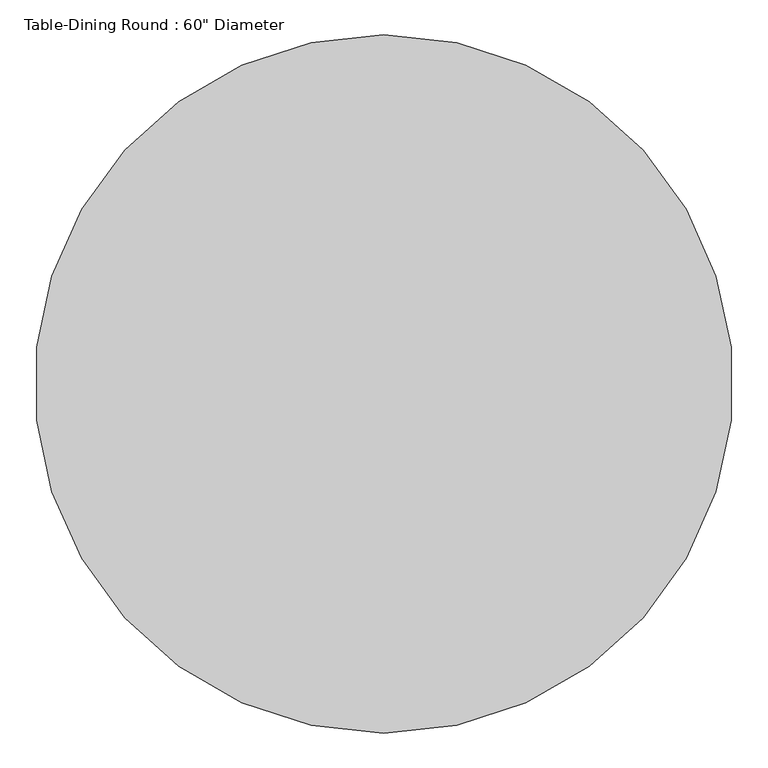
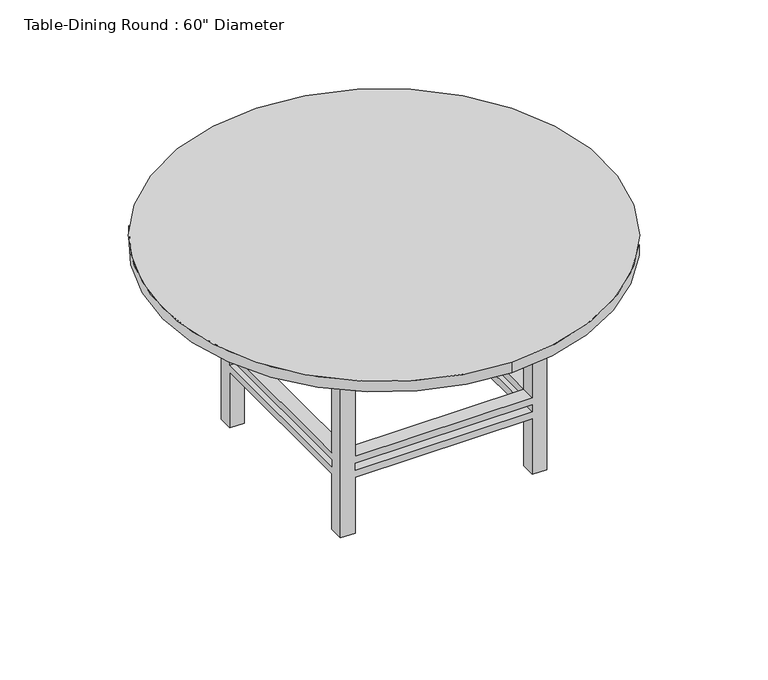
"""IFC4 building model written with IfcOpenShell, lengths in millimetres: furniture geometry."""

from ifc_helpers import new_model, si_unit, point, frame, frame_2d, origin, place, context, project, spatial, polyline, circle_curve, trimmed, segment, composite_curve, outline, extrude, faceted_brep, source, transform, mapped, element, save


def furniture_720490b2(model_context):
    return source(origin(), model_context, "Body", "SolidModel", [
        faceted_brep([(-201.1180328, 170.7213115, 723.9), (-251.9180328, 170.7213115, 723.9), (-251.9180328, 119.9213115, 723.9), (-201.1180328, 119.9213115, 723.9), (408.4819672, 170.7213115, 723.9), (408.4819672, 119.9213115, 723.9), (459.2819672, 119.9213115, 723.9), (459.2819672, 170.7213115, 723.9), (408.4819672, -540.4786885, 723.9), (459.2819672, -540.4786885, 723.9), (459.2819672, -489.6786885, 723.9), (408.4819672, -489.6786885, 723.9), (-201.1180328, -540.4786885, 723.9), (-201.1180328, -489.6786885, 723.9), (-251.9180328, -489.6786885, 723.9), (-251.9180328, -540.4786885, 723.9), (-201.1180328, 170.7213115, 0.0), (-201.1180328, 119.9213115, 0.0), (-251.9180328, 119.9213115, 0.0), (-251.9180328, 170.7213115, 0.0), (408.4819672, 170.7213115, 0.0), (459.2819672, 170.7213115, 0.0), (459.2819672, 119.9213115, 0.0), (408.4819672, 119.9213115, 0.0), (408.4819672, -540.4786885, 0.0), (408.4819672, -489.6786885, 0.0), (459.2819672, -489.6786885, 0.0), (459.2819672, -540.4786885, 0.0), (-201.1180328, -540.4786885, 0.0), (-251.9180328, -540.4786885, 0.0), (-251.9180328, -489.6786885, 0.0), (-201.1180328, -489.6786885, 0.0), (-201.1180328, 170.7213115, 279.4), (408.4819672, 170.7213115, 279.4), (408.4819672, 170.7213115, 203.2), (-201.1180328, 170.7213115, 203.2), (408.4819672, 170.7213115, 228.6), (408.4819672, 170.7213115, 254.0), (-201.1180328, 170.7213115, 254.0), (-201.1180328, 170.7213115, 228.6), (-251.9180328, 119.9213115, 203.2), (-251.9180328, -489.6786885, 203.2), (-251.9180328, -489.6786885, 279.4), (-251.9180328, 119.9213115, 279.4), (-251.9180328, 119.9213115, 228.6), (-251.9180328, 119.9213115, 254.0), (-251.9180328, -489.6786885, 254.0), (-251.9180328, -489.6786885, 228.6), (-201.1180328, 119.9213115, 279.4), (-201.1180328, 119.9213115, 203.2), (-201.1180328, 119.9213115, 228.6), (-201.1180328, 119.9213115, 254.0), (408.4819672, 119.9213115, 279.4), (408.4819672, 119.9213115, 203.2), (408.4819672, 119.9213115, 228.6), (408.4819672, 119.9213115, 254.0), (459.2819672, 119.9213115, 279.4), (459.2819672, 119.9213115, 203.2), (459.2819672, 119.9213115, 228.6), (459.2819672, 119.9213115, 254.0), (459.2819672, -489.6786885, 279.4), (459.2819672, -489.6786885, 203.2), (459.2819672, -489.6786885, 228.6), (459.2819672, -489.6786885, 254.0), (408.4819672, -540.4786885, 279.4), (-201.1180328, -540.4786885, 279.4), (-201.1180328, -540.4786885, 203.2), (408.4819672, -540.4786885, 203.2), (-201.1180328, -540.4786885, 228.6), (-201.1180328, -540.4786885, 254.0), (408.4819672, -540.4786885, 254.0), (408.4819672, -540.4786885, 228.6), (408.4819672, -489.6786885, 279.4), (408.4819672, -489.6786885, 203.2), (408.4819672, -489.6786885, 228.6), (408.4819672, -489.6786885, 254.0), (-201.1180328, -489.6786885, 279.4), (-201.1180328, -489.6786885, 203.2), (-201.1180328, -489.6786885, 228.6), (-201.1180328, -489.6786885, 254.0)], [[[0, 1, 2, 3]], [[4, 5, 6, 7]], [[8, 9, 10, 11]], [[12, 13, 14, 15]], [[16, 17, 18, 19]], [[20, 21, 22, 23]], [[24, 25, 26, 27]], [[28, 29, 30, 31]], [[1, 0, 32, 33, 4, 7, 21, 20, 34, 35, 16, 19], [36, 37, 38, 39]], [[2, 1, 19, 18, 40, 41, 30, 29, 15, 14, 42, 43], [44, 45, 46, 47]], [[3, 2, 43, 48]], [[18, 17, 49, 40]], [[44, 50, 51, 45]], [[0, 3, 48, 32]], [[17, 16, 35, 49]], [[50, 39, 38, 51]], [[5, 4, 33, 52]], [[20, 23, 53, 34]], [[36, 54, 55, 37]], [[6, 5, 52, 56]], [[23, 22, 57, 53]], [[54, 58, 59, 55]], [[21, 7, 6, 56, 60, 10, 9, 27, 26, 61, 57, 22], [62, 63, 59, 58]], [[27, 9, 8, 64, 65, 12, 15, 29, 28, 66, 67, 24], [68, 69, 70, 71]], [[11, 10, 60, 72]], [[26, 25, 73, 61]], [[62, 74, 75, 63]], [[8, 11, 72, 64]], [[25, 24, 67, 73]], [[74, 71, 70, 75]], [[13, 12, 65, 76]], [[28, 31, 77, 66]], [[68, 78, 79, 69]], [[14, 13, 76, 42]], [[31, 30, 41, 77]], [[78, 47, 46, 79]], [[54, 74, 62, 58]], [[74, 78, 68, 71]], [[78, 50, 44, 47]], [[50, 54, 36, 39]], [[53, 49, 35, 34]], [[49, 77, 41, 40]], [[77, 73, 67, 66]], [[73, 53, 57, 61]], [[74, 54, 53, 73]], [[78, 74, 73, 77]], [[50, 78, 77, 49]], [[54, 50, 49, 53]], [[52, 72, 60, 56]], [[72, 76, 65, 64]], [[76, 48, 43, 42]], [[48, 52, 33, 32]], [[55, 51, 38, 37]], [[51, 79, 46, 45]], [[79, 75, 70, 69]], [[75, 55, 59, 63]], [[72, 52, 55, 75]], [[76, 72, 75, 79]], [[48, 76, 79, 51]], [[52, 48, 51, 55]]]),
        extrude(outline(polyline([(484.6819672, 196.1213115), (484.6819672, -565.8786885), (-277.3180328, -565.8786885), (-277.3180328, 196.1213115), (484.6819672, 196.1213115)]), holes=[polyline([(459.2819672, 170.7213115), (-251.9180328, 170.7213115), (-251.9180328, -540.4786885), (459.2819672, -540.4786885), (459.2819672, 170.7213115)])]), frame((0.0, 0.0, 647.7), z_axis=(0.0, 0.0, 1.0), x_axis=(1.0, 0.0, 0.0)), (0.0, 0.0, 1.0), 76.2),
        extrude(outline(composite_curve([segment(trimmed(circle_curve(frame_2d((103.6819672, -184.8786885)), 762.0), [point((103.6819672, -946.8786885))], [point((103.6819672, 577.1213115))], False, "CARTESIAN"), True, "CONTINUOUS"), segment(trimmed(circle_curve(frame_2d((103.6819672, -184.8786885)), 762.0), [point((103.6819672, 577.1213115))], [point((103.6819672, -946.8786885))], False, "CARTESIAN"), True, "CONTINUOUS")], self_intersect=False)), frame((0.0, 0.0, 723.9), z_axis=(0.0, 0.0, 1.0), x_axis=(1.0, 0.0, 0.0)), (0.0, 0.0, 1.0), 38.1),
    ])


if __name__ == "__main__":
    model = new_model("IFC4")
    model_context = context("Model", 3, world=origin())
    ifc_project = project(units=[si_unit("LENGTHUNIT", "METRE", prefix="MILLI")], contexts=[model_context])
    site = spatial("IfcSite", under=ifc_project)
    building = spatial("IfcBuilding", under=site)
    placement = place(None, origin())
    furniture_shape = furniture_720490b2(model_context)
    element("IfcFurniture", 1, ObjectType="Table-Dining Round : 60\" Diameter", at=placement, inside=building, context=model_context, shape_type="MappedRepresentation", body=[
        mapped(furniture_shape, transform((0.0, 0.0, 0.0), x_axis=(1.0, 0.0, 0.0), y_axis=(0.0, 1.0, 0.0), z_axis=(0.0, 0.0, 1.0))),
    ])
    save(model, "model.ifc")

# Revit data of these elements
# Type "Table-Dining Round : 60\" Diameter"
#   Assembly Code = "E2020200"
#   Diameter = 5' - 0"
#   Height = 2' - 6"
#   Base Material = Pine
#   Top Material = Laminate, Linen, Matte
#   Default Elevation = 0
# Element 1 (IfcFurniture, "Table-Dining Round : 60\" Diameter")
#   Materials on its faces: "Pine", "Laminate, Linen, Matte"
# Materials
#   "Pine": class "Wood", colour RGB 223 192 134, transparency 0, Description = "Pinus Echinata", Cost = 0
#   "Laminate, Linen, Matte": class "Plastic", colour RGB 249 239 230, transparency 0, Description = "Plastic Laminate - Linen, Matte", Cost = 0
